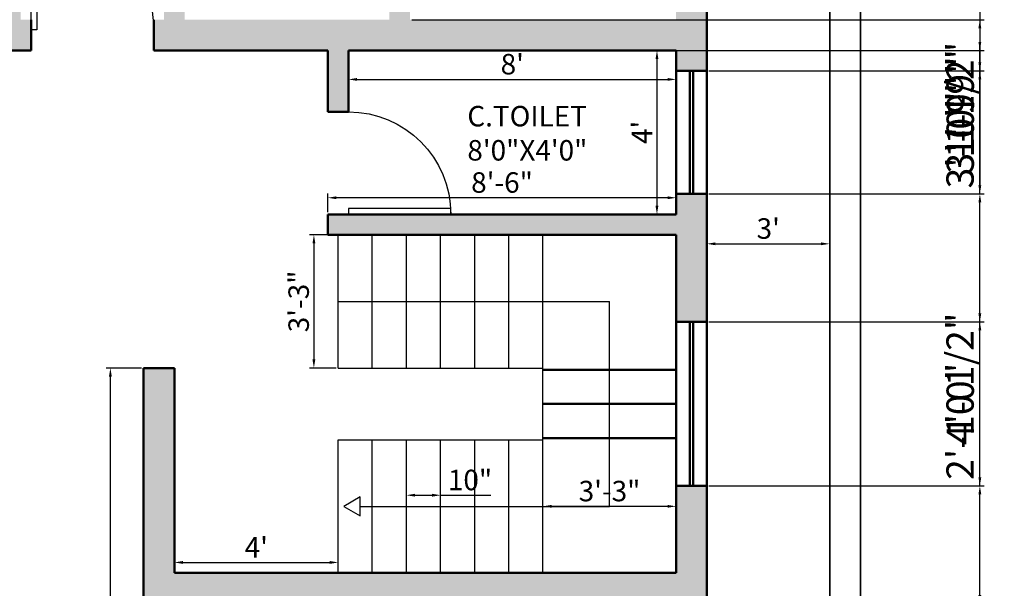
# Model space of a CAD drawing. Units: inches. Extents: x 2442 to 3851, y 589 to 2836.
# Tile 16 of 22: x 2847 to 3136, y 2397 to 2563. Entities that reach past the tile are written whole.
import ezdxf

# ---------------------------------------------------------------- set-up
doc = ezdxf.new("R2010")
doc.units = ezdxf.units.IN
for name, color, linetype, lineweight in [('A-ANNO-DIMS', 2, 'Continuous', 18), ('A-AREA-IDEN', 7, 'Continuous', 18), ('A-DOOR', 4, 'Continuous', 25), ('A-FLOR-STRS', 3, 'Continuous', 25), ('A-WALL', 7, 'Continuous', 50), ('A-WALL-PATT', 8, 'Continuous', 13), ('C-PROP', 7, 'Continuous', 35)]:
    doc.layers.add(name, color=color, linetype=linetype, lineweight=lineweight)
doc.styles.get("Standard").update_dxf_attribs({"font": 'arial.ttf'})
doc.dimstyles.new('ISO-25', dxfattribs={"dimtxt": 8, "dimasz": 2.5, "dimexe": 1.25, "dimexo": 0.625, "dimtad": 1, "dimlunit": 3, "dimtxsty": 'Standard', "dimcen": 2.5, "dimadec": 0, "dimazin": 0, "dimtfac": 1, "dimtmove": 0, "dimatfit": 3, "dimfxl": 1, "dimarcsym": 0})

# ---------------------------------------------------------------- blocks, each defined once
blk = doc.blocks.new('*U23')
for p, q in [((0, 0), (0, -6)), ((36, 0), (36, -6))]:
    blk.add_line(p, q)
blk.add_lwpolyline([(0, 0), (0, 36), (1.75, 36), (1.75, 0)], close=True)
blk.add_arc((0, 0), 36, 0, 90)
blk = doc.blocks.new('*U24')
for p, q in [((0, 0), (0, -6)), ((30, 0), (30, -6))]:
    blk.add_line(p, q)
blk.add_lwpolyline([(0, 0), (0, 30), (1.75, 30), (1.75, 0)], close=True)
blk.add_arc((0, 0), 30, 0, 90)
blk = doc.blocks.new('*D42')
at = {"layer": 'A-ANNO-DIMS', "color": 0, "lineweight": -2, "transparency": 16777216}
for p, q in [((3048.6, 2498.21), (3048.6, 2498.83)), ((3084.6, 2498.21), (3084.6, 2498.83)), ((3051.1, 2497.58), (3082.1, 2497.58))]:
    blk.add_line(p, q, dxfattribs=at)
at = {"layer": 'A-ANNO-DIMS', "color": 0, "transparency": 16777216}
for points in [[(3051.1, 2498), (3051.1, 2497.17), (3048.6, 2497.58)], [(3082.1, 2498), (3082.1, 2497.17), (3084.6, 2497.58)]]:
    blk.add_solid(points, dxfattribs=at)
at = {"layer": 'Defpoints', "color": 0, "transparency": 16777216}
for p in [(3048.6, 2497.58), (3084.6, 2497.58), (3084.6, 2497.58)]:
    blk.add_point(p, dxfattribs=at)
at = {"layer": 'A-ANNO-DIMS', "color": 0, "transparency": 16777216, "insert": (3066.6, 2501.28), "char_height": 6, "attachment_point": 5}
blk.add_mtext("3'", dxfattribs=at)
blk = doc.blocks.new('*D52')
at = {"layer": 'A-ANNO-DIMS', "color": 0, "lineweight": -2, "transparency": 16777216}
for p, q in [((2943.6, 2553.58), (2943.6, 2544.47)), ((3039.6, 2553.58), (3039.6, 2544.47)), ((2946.1, 2545.72), (3037.1, 2545.72))]:
    blk.add_line(p, q, dxfattribs=at)
at = {"layer": 'A-ANNO-DIMS', "color": 0, "transparency": 16777216}
for points in [[(2946.1, 2546.14), (2946.1, 2545.31), (2943.6, 2545.72)], [(3037.1, 2546.14), (3037.1, 2545.31), (3039.6, 2545.72)]]:
    blk.add_solid(points, dxfattribs=at)
at = {"layer": 'Defpoints', "color": 0, "transparency": 16777216}
for p in [(2943.6, 2554.21), (3039.6, 2554.21), (3039.6, 2545.72)]:
    blk.add_point(p, dxfattribs=at)
at = {"layer": 'A-ANNO-DIMS', "color": 0, "transparency": 16777216, "insert": (2991.6, 2549.41), "char_height": 6, "attachment_point": 5}
blk.add_mtext("8'", dxfattribs=at)
blk = doc.blocks.new('*D53')
at = {"layer": 'A-ANNO-DIMS', "color": 0, "lineweight": -2, "transparency": 16777216}
for p, q in [((3038.97, 2554.21), (3032.75, 2554.21)), ((3034, 2551.71), (3034, 2508.71)), ((3038.97, 2506.21), (3032.75, 2506.21))]:
    blk.add_line(p, q, dxfattribs=at)
at = {"layer": 'A-ANNO-DIMS', "color": 0, "transparency": 16777216}
for points in [[(3033.58, 2551.71), (3034.41, 2551.71), (3034, 2554.21)], [(3033.58, 2508.71), (3034.41, 2508.71), (3034, 2506.21)]]:
    blk.add_solid(points, dxfattribs=at)
at = {"layer": 'Defpoints', "color": 0, "transparency": 16777216}
for p in [(3039.6, 2554.21), (3034, 2506.21), (3039.6, 2506.21)]:
    blk.add_point(p, dxfattribs=at)
at = {"layer": 'A-ANNO-DIMS', "color": 0, "transparency": 16777216, "insert": (3030.37, 2530.21), "char_height": 6, "attachment_point": 5, "rotation": 90}
blk.add_mtext("4'", dxfattribs=at)
blk = doc.blocks.new('*D55')
at = {"layer": 'A-ANNO-DIMS', "color": 0, "lineweight": -2, "transparency": 16777216}
for p, q in [((2882.97, 2461.21), (2872.6, 2461.21)), ((2873.85, 2259.71), (2873.85, 2458.71)), ((2882.97, 2257.21), (2872.6, 2257.21))]:
    blk.add_line(p, q, dxfattribs=at)
at = {"layer": 'A-ANNO-DIMS', "color": 0, "transparency": 16777216}
for points in [[(2873.44, 2458.71), (2874.27, 2458.71), (2873.85, 2461.21)], [(2873.44, 2259.71), (2874.27, 2259.71), (2873.85, 2257.21)]]:
    blk.add_solid(points, dxfattribs=at)
at = {"layer": 'Defpoints', "color": 0, "transparency": 16777216}
for p in [(2873.85, 2461.21), (2883.6, 2461.21), (2883.6, 2257.21)]:
    blk.add_point(p, dxfattribs=at)
at = {"layer": 'A-ANNO-DIMS', "color": 0, "transparency": 16777216, "insert": (2870.22, 2359.21), "char_height": 6, "attachment_point": 5, "rotation": 90}
blk.add_mtext("17'", dxfattribs=at)
blk = doc.blocks.new('*D68')
at = {"layer": 'A-ANNO-DIMS', "color": 0, "lineweight": -2, "transparency": 16777216}
for p, q in [((2937.6, 2506.83), (2937.6, 2512.32)), ((3037.1, 2511.07), (2940.1, 2511.07)), ((3039.6, 2506.83), (3039.6, 2512.32))]:
    blk.add_line(p, q, dxfattribs=at)
at = {"layer": 'A-ANNO-DIMS', "color": 0, "transparency": 16777216}
for points in [[(2940.1, 2511.49), (2940.1, 2510.65), (2937.6, 2511.07)], [(3037.1, 2511.49), (3037.1, 2510.65), (3039.6, 2511.07)]]:
    blk.add_solid(points, dxfattribs=at)
at = {"layer": 'Defpoints', "color": 0, "transparency": 16777216}
for p in [(2937.6, 2511.07), (2937.6, 2506.21), (3039.6, 2506.21)]:
    blk.add_point(p, dxfattribs=at)
at = {"layer": 'A-ANNO-DIMS', "color": 0, "transparency": 16777216, "insert": (2988.6, 2514.76), "char_height": 6, "attachment_point": 5}
blk.add_mtext('8\'-6"', dxfattribs=at)
blk = doc.blocks.new('*D69')
at = {"layer": 'A-ANNO-DIMS', "color": 0, "lineweight": -2, "transparency": 16777216}
for p, q in [((2892.6, 2401.83), (2892.6, 2405.53)), ((2895.1, 2404.28), (2938.1, 2404.28)), ((2940.6, 2401.83), (2940.6, 2405.53))]:
    blk.add_line(p, q, dxfattribs=at)
at = {"layer": 'A-ANNO-DIMS', "color": 0, "transparency": 16777216}
for points in [[(2895.1, 2404.7), (2895.1, 2403.86), (2892.6, 2404.28)], [(2938.1, 2404.7), (2938.1, 2403.86), (2940.6, 2404.28)]]:
    blk.add_solid(points, dxfattribs=at)
at = {"layer": 'Defpoints', "color": 0, "transparency": 16777216}
for p in [(2940.6, 2404.28), (2892.6, 2401.21), (2940.6, 2401.21)]:
    blk.add_point(p, dxfattribs=at)
at = {"layer": 'A-ANNO-DIMS', "color": 0, "transparency": 16777216, "insert": (2916.6, 2407.91), "char_height": 6, "attachment_point": 5}
blk.add_mtext("4'", dxfattribs=at)
blk = doc.blocks.new('*D70')
at = {"layer": 'A-ANNO-DIMS', "color": 0, "lineweight": -2, "transparency": 16777216}
for p, q in [((2939.97, 2500.21), (2932.23, 2500.21)), ((2933.48, 2497.71), (2933.48, 2463.71)), ((2939.97, 2461.21), (2932.23, 2461.21))]:
    blk.add_line(p, q, dxfattribs=at)
at = {"layer": 'A-ANNO-DIMS', "color": 0, "transparency": 16777216}
for points in [[(2933.06, 2497.71), (2933.9, 2497.71), (2933.48, 2500.21)], [(2933.06, 2463.71), (2933.9, 2463.71), (2933.48, 2461.21)]]:
    blk.add_solid(points, dxfattribs=at)
at = {"layer": 'Defpoints', "color": 0, "transparency": 16777216}
for p in [(2940.6, 2500.21), (2933.48, 2461.21), (2940.6, 2461.21)]:
    blk.add_point(p, dxfattribs=at)
at = {"layer": 'A-ANNO-DIMS', "color": 0, "transparency": 16777216, "insert": (2929.79, 2480.71), "char_height": 6, "attachment_point": 5, "rotation": 90}
blk.add_mtext('3\'-3"', dxfattribs=at)
blk = doc.blocks.new('*D71')
at = {"layer": 'A-ANNO-DIMS', "color": 0, "lineweight": -2, "transparency": 16777216}
for p, q in [((3000.6, 2421.33), (3000.6, 2421.96)), ((3003.1, 2420.71), (3037.1, 2420.71)), ((3039.6, 2421.33), (3039.6, 2421.96))]:
    blk.add_line(p, q, dxfattribs=at)
at = {"layer": 'A-ANNO-DIMS', "color": 0, "transparency": 16777216}
for points in [[(3003.1, 2421.12), (3003.1, 2420.29), (3000.6, 2420.71)], [(3037.1, 2421.12), (3037.1, 2420.29), (3039.6, 2420.71)]]:
    blk.add_solid(points, dxfattribs=at)
at = {"layer": 'Defpoints', "color": 0, "transparency": 16777216}
for p in [(3000.6, 2420.71), (3039.6, 2420.71), (3039.6, 2420.71)]:
    blk.add_point(p, dxfattribs=at)
at = {"layer": 'A-ANNO-DIMS', "color": 0, "transparency": 16777216, "insert": (3020.1, 2424.4), "char_height": 6, "attachment_point": 5}
blk.add_mtext('3\'-3"', dxfattribs=at)
blk = doc.blocks.new('*D72')
at = {"layer": 'A-ANNO-DIMS', "color": 0, "lineweight": -2, "transparency": 16777216}
for p, q in [((2960.6, 2424.59), (2960.6, 2425.21)), ((2963.1, 2423.96), (2968.1, 2423.96)), ((2970.6, 2424.59), (2970.6, 2425.21)), ((2970.6, 2423.96), (2985.34, 2423.96))]:
    blk.add_line(p, q, dxfattribs=at)
at = {"layer": 'A-ANNO-DIMS', "color": 0, "transparency": 16777216}
for points in [[(2963.1, 2424.38), (2963.1, 2423.55), (2960.6, 2423.96)], [(2968.1, 2424.38), (2968.1, 2423.55), (2970.6, 2423.96)]]:
    blk.add_solid(points, dxfattribs=at)
at = {"layer": 'Defpoints', "color": 0, "transparency": 16777216}
for p in [(2960.6, 2423.96), (2970.6, 2423.96), (2970.6, 2423.96)]:
    blk.add_point(p, dxfattribs=at)
at = {"layer": 'A-ANNO-DIMS', "color": 0, "transparency": 16777216, "insert": (2979.22, 2427.65), "char_height": 6, "attachment_point": 5}
blk.add_mtext('10"', dxfattribs=at)
blk = doc.blocks.new('*D191')
at = {"layer": 'A-ANNO-DIMS', "color": 0, "lineweight": -2, "transparency": 16777216}
for p, q in [((3128.6, 2426.71), (3128.6, 2476.72)), ((3049.22, 2426.71), (3129.85, 2426.71)), ((3128.6, 2394.71), (3128.6, 2424.21)), ((3049.22, 2392.21), (3129.85, 2392.21))]:
    blk.add_line(p, q, dxfattribs=at)
at = {"layer": 'A-ANNO-DIMS', "color": 0, "transparency": 16777216}
for points in [[(3128.18, 2424.21), (3129.02, 2424.21), (3128.6, 2426.71)], [(3128.18, 2394.71), (3129.02, 2394.71), (3128.6, 2392.21)]]:
    blk.add_solid(points, dxfattribs=at)
at = {"layer": 'Defpoints', "color": 0, "transparency": 16777216}
for p in [(3048.6, 2426.71), (3128.6, 2426.71), (3048.6, 2392.21)]:
    blk.add_point(p, dxfattribs=at)
at = {"layer": 'A-ANNO-DIMS', "color": 0, "transparency": 16777216, "insert": (3123.84, 2452.96), "char_height": 8, "attachment_point": 5, "rotation": 90}
blk.add_mtext('2\'-10 1/2"', dxfattribs=at)
blk = doc.blocks.new('*D192')
at = {"layer": 'A-ANNO-DIMS', "color": 0, "lineweight": -2, "transparency": 16777216}
for p, q in [((3049.22, 2474.71), (3129.85, 2474.71)), ((3128.6, 2429.21), (3128.6, 2472.21)), ((3049.22, 2426.71), (3129.85, 2426.71))]:
    blk.add_line(p, q, dxfattribs=at)
at = {"layer": 'A-ANNO-DIMS', "color": 0, "transparency": 16777216}
for points in [[(3128.18, 2472.21), (3129.02, 2472.21), (3128.6, 2474.71)], [(3128.18, 2429.21), (3129.02, 2429.21), (3128.6, 2426.71)]]:
    blk.add_solid(points, dxfattribs=at)
at = {"layer": 'Defpoints', "color": 0, "transparency": 16777216}
for p in [(3048.6, 2474.71), (3128.6, 2474.71), (3048.6, 2426.71)]:
    blk.add_point(p, dxfattribs=at)
at = {"layer": 'A-ANNO-DIMS', "color": 0, "transparency": 16777216, "insert": (3123.89, 2450.71), "char_height": 8, "attachment_point": 5, "rotation": 90}
blk.add_mtext('4\'-0"', dxfattribs=at)
blk = doc.blocks.new('*D193')
at = {"layer": 'A-ANNO-DIMS', "color": 0, "lineweight": -2, "transparency": 16777216}
for p, q in [((3128.6, 2512.21), (3128.6, 2555.86)), ((3049.22, 2512.21), (3129.85, 2512.21)), ((3128.6, 2477.21), (3128.6, 2509.71)), ((3049.22, 2474.71), (3129.85, 2474.71))]:
    blk.add_line(p, q, dxfattribs=at)
at = {"layer": 'A-ANNO-DIMS', "color": 0, "transparency": 16777216}
for points in [[(3128.18, 2509.71), (3129.02, 2509.71), (3128.6, 2512.21)], [(3128.18, 2477.21), (3129.02, 2477.21), (3128.6, 2474.71)]]:
    blk.add_solid(points, dxfattribs=at)
at = {"layer": 'Defpoints', "color": 0, "transparency": 16777216}
for p in [(3048.6, 2512.21), (3128.6, 2512.21), (3048.6, 2474.71)]:
    blk.add_point(p, dxfattribs=at)
at = {"layer": 'A-ANNO-DIMS', "color": 0, "transparency": 16777216, "insert": (3123.83, 2535.28), "char_height": 8, "attachment_point": 5, "rotation": 90}
blk.add_mtext('3\'-1 1/2"', dxfattribs=at)
blk = doc.blocks.new('*D196')
at = {"layer": 'A-ANNO-DIMS', "color": 0, "lineweight": -2, "transparency": 16777216}
for p, q in [((3049.22, 2569.21), (3129.85, 2569.21)), ((3128.6, 2566.71), (3128.6, 2550.71)), ((3049.22, 2548.21), (3129.85, 2548.21)), ((3128.6, 2548.21), (3128.6, 2523.94))]:
    blk.add_line(p, q, dxfattribs=at)
at = {"layer": 'A-ANNO-DIMS', "color": 0, "transparency": 16777216}
for points in [[(3128.18, 2566.71), (3129.02, 2566.71), (3128.6, 2569.21)], [(3128.18, 2550.71), (3129.02, 2550.71), (3128.6, 2548.21)]]:
    blk.add_solid(points, dxfattribs=at)
at = {"layer": 'Defpoints', "color": 0, "transparency": 16777216}
for p in [(3048.6, 2569.21), (3048.6, 2548.21), (3128.6, 2548.21)]:
    blk.add_point(p, dxfattribs=at)
at = {"layer": 'A-ANNO-DIMS', "color": 0, "transparency": 16777216, "insert": (3123.89, 2534.83), "char_height": 8, "attachment_point": 5, "rotation": 90}
blk.add_mtext('1\'-9"', dxfattribs=at)
blk = doc.blocks.new('*D197')
at = {"layer": 'A-ANNO-DIMS', "color": 0, "lineweight": -2, "transparency": 16777216}
for p, q in [((3049.22, 2548.21), (3129.85, 2548.21)), ((3128.6, 2545.71), (3128.6, 2514.71)), ((3049.22, 2512.21), (3129.85, 2512.21))]:
    blk.add_line(p, q, dxfattribs=at)
at = {"layer": 'A-ANNO-DIMS', "color": 0, "transparency": 16777216}
for points in [[(3128.18, 2545.71), (3129.02, 2545.71), (3128.6, 2548.21)], [(3128.18, 2514.71), (3129.02, 2514.71), (3128.6, 2512.21)]]:
    blk.add_solid(points, dxfattribs=at)
at = {"layer": 'Defpoints', "color": 0, "transparency": 16777216}
for p in [(3048.6, 2548.21), (3048.6, 2512.21), (3128.6, 2512.21)]:
    blk.add_point(p, dxfattribs=at)
at = {"layer": 'A-ANNO-DIMS', "color": 0, "transparency": 16777216, "insert": (3123.89, 2530.21), "char_height": 8, "attachment_point": 5, "rotation": 90}
blk.add_mtext('3\'-0"', dxfattribs=at)
blk = doc.blocks.new('*D215')
at = {"layer": 'A-ANNO-DIMS', "color": 0, "lineweight": -2, "transparency": 16777216}
for p, q in [((2962.22, 2563.21), (3129.85, 2563.21)), ((3128.6, 2560.71), (3128.6, 2556.71)), ((2944.22, 2554.21), (3129.85, 2554.21)), ((3128.6, 2554.21), (3128.6, 2529.19))]:
    blk.add_line(p, q, dxfattribs=at)
at = {"layer": 'A-ANNO-DIMS', "color": 0, "transparency": 16777216}
for points in [[(3128.18, 2560.71), (3129.02, 2560.71), (3128.6, 2563.21)], [(3128.18, 2556.71), (3129.02, 2556.71), (3128.6, 2554.21)]]:
    blk.add_solid(points, dxfattribs=at)
at = {"layer": 'Defpoints', "color": 0, "transparency": 16777216}
for p in [(2961.6, 2563.21), (2943.6, 2554.21), (3128.6, 2554.21)]:
    blk.add_point(p, dxfattribs=at)
at = {"layer": 'A-ANNO-DIMS', "color": 0, "transparency": 16777216, "insert": (3123.89, 2540.45), "char_height": 8, "attachment_point": 5, "rotation": 90}
blk.add_mtext('0\'-9"', dxfattribs=at)

msp = doc.modelspace()

# ---------------------------------------------------------------- hatches: boundary and pattern name
at = {"layer": 'A-WALL-PATT'}
h = msp.add_hatch(color=256, dxfattribs=at)
h.dxf.hatch_style = 1
h.paths.add_polyline_path([(2640.599, 2713.208), (2640.599, 2719.208), (2640.599, 2722.208), (2538.599, 2722.208), (2538.599, 2657.708), (2547.599, 2657.708), (2547.599, 2713.208)])
h.paths.add_polyline_path([(2700.599, 2737.208), (2730.599, 2737.208), (2730.599, 2746.208), (2700.599, 2746.208), (2700.599, 2782.208), (2691.599, 2782.208), (2691.599, 2722.208), (2670.599, 2722.208), (2670.599, 2719.208), (2670.599, 2713.208), (2691.599, 2713.208), (2691.599, 2608.208), (2799.599, 2608.208), (2799.599, 2614.208), (2799.599, 2617.208), (2700.599, 2617.208)])
h.paths.add_polyline_path([(2838.599, 2737.208), (2838.599, 2617.208), (2835.599, 2617.208), (2835.599, 2614.208), (2835.599, 2608.208), (2838.599, 2608.208), (2838.599, 2554.208), (2850.599, 2554.208), (2850.599, 2560.208), (2850.599, 2563.208), (2847.599, 2563.208), (2847.599, 2737.208), (2850.599, 2737.208), (2850.599, 2746.208), (2796.599, 2746.208), (2796.599, 2737.208)])
h.paths.add_polyline_path([(2898.599, 2746.208), (2898.599, 2737.208), (2967.599, 2737.208), (2967.599, 2746.208)])
h.paths.add_polyline_path([(3048.599, 2746.208), (3015.599, 2746.208), (3015.599, 2737.208), (3039.599, 2737.208), (3039.599, 2665.208), (3048.599, 2665.208)])
h.paths.add_polyline_path([(3039.599, 2611.208), (3039.599, 2605.208), (3048.599, 2605.208), (3048.599, 2617.208), (2946.599, 2617.208), (2946.599, 2611.208)])
h.paths.add_polyline_path([(2961.599, 2563.208), (2961.599, 2581.208), (2955.599, 2581.208), (2955.599, 2563.208), (2895.599, 2563.208), (2895.599, 2611.208), (2916.599, 2611.208), (2916.599, 2617.208), (2889.599, 2617.208), (2889.599, 2563.208), (2886.599, 2563.208), (2886.599, 2554.208), (2937.599, 2554.208), (2937.599, 2536.208), (2943.599, 2536.208), (2943.599, 2554.208), (3039.599, 2554.208), (3039.599, 2548.208), (3048.599, 2548.208), (3048.599, 2569.208), (3039.599, 2569.208), (3039.599, 2563.208)])
h.paths.add_polyline_path([(2538.599, 2521.208), (2547.599, 2521.208), (2547.599, 2545.208), (2694.599, 2545.208), (2694.599, 2542.208), (2697.599, 2542.208), (2703.599, 2542.208), (2703.599, 2554.208), (2547.599, 2554.208), (2547.599, 2609.708), (2538.599, 2609.708)])
h.paths.add_polyline_path([(2538.599, 2368.208), (2547.599, 2368.208), (2547.599, 2392.208), (2694.599, 2392.208), (2694.599, 2344.208), (2703.599, 2344.208), (2703.599, 2506.208), (2697.599, 2506.208), (2694.599, 2506.208), (2694.599, 2401.208), (2547.599, 2401.208), (2547.599, 2473.208), (2538.599, 2473.208)])
h.paths.add_polyline_path([(2547.599, 2287.208), (2553.599, 2287.208), (2553.599, 2293.208), (2553.599, 2296.208), (2547.599, 2296.208), (2547.599, 2320.208), (2538.599, 2320.208), (2538.599, 2191.208), (2547.599, 2191.208)])
h.paths.add_polyline_path([(2703.599, 2296.208), (2670.599, 2296.208), (2670.599, 2287.208), (2694.599, 2287.208), (2694.599, 2248.208), (2733.599, 2248.208), (2733.599, 2257.208), (2703.599, 2257.208)])
h.paths.add_polyline_path([(2593.599, 2287.208), (2604.599, 2287.208), (2604.599, 2296.208), (2593.599, 2296.208)])
h.paths.add_polyline_path([(2799.599, 2248.208), (2799.599, 2257.208), (2775.599, 2257.208), (2775.599, 2248.208)])
h.paths.add_polyline_path([(2892.599, 2248.208), (2892.599, 2287.208), (2883.599, 2287.208), (2883.599, 2257.208), (2865.599, 2257.208), (2865.599, 2248.208)])
h.paths.add_polyline_path([(2883.599, 2353.208), (2892.599, 2353.208), (2892.599, 2392.208), (3048.599, 2392.208), (3048.599, 2426.708), (3039.599, 2426.708), (3039.599, 2401.208), (2892.599, 2401.208), (2892.599, 2461.208), (2883.599, 2461.208)])
h.paths.add_polyline_path([(3039.599, 2474.708), (3048.599, 2474.708), (3048.599, 2512.208), (3039.599, 2512.208), (3039.599, 2506.208), (2937.599, 2506.208), (2937.599, 2500.208), (3039.599, 2500.208)])

# ---------------------------------------------------------------- linework, layer by layer
at = {"layer": 'A-FLOR-STRS'}
for p, q in [((2940.599, 2461.208), (2940.599, 2500.208)), ((2950.599, 2461.208), (2950.599, 2500.208)), ((2960.599, 2461.208), (2960.599, 2500.208)), ((2970.599, 2461.208), (2970.599, 2500.208)), ((2980.599, 2461.208), (2980.599, 2500.208)), ((2990.599, 2461.208), (2990.599, 2500.208)), ((3000.599, 2440.208), (3000.599, 2500.208)), ((2940.599, 2480.708), (3020.099, 2480.708)), ((3020.099, 2420.708), (3020.099, 2480.708)), ((2940.599, 2461.208), (3000.599, 2461.208)), ((2940.599, 2440.208), (3000.599, 2440.208)), ((2947.056, 2420.708), (3020.099, 2420.708))]:
    msp.add_line(p, q, dxfattribs=at)
at = {"layer": 'A-FLOR-STRS', "ltscale": 0.5}
for p, q in [((2940.599, 2401.208), (2940.599, 2440.208)), ((2950.599, 2401.208), (2950.599, 2440.208)), ((2960.599, 2401.208), (2960.599, 2440.208)), ((2970.599, 2401.208), (2970.599, 2440.208)), ((2980.599, 2401.208), (2980.599, 2440.208)), ((2990.599, 2401.208), (2990.599, 2440.208)), ((3000.599, 2401.208), (3000.599, 2440.208))]:
    msp.add_line(p, q, dxfattribs=at)
at = {"layer": 'A-FLOR-STRS'}
msp.add_lwpolyline([(2942.213, 2420.708), (2947.056, 2417.911), (2947.056, 2423.504)], close=True, dxfattribs=at)
at = {"layer": 'A-WALL'}
for p, q in [((3048.599, 2392.208), (3048.599, 2746.208)), ((2850.599, 2554.208), (2850.599, 2563.208)), ((2886.599, 2554.208), (2886.599, 2563.208)), ((2838.599, 2554.208), (2850.599, 2554.208)), ((2886.599, 2554.208), (2937.599, 2554.208)), ((2937.599, 2536.208), (2937.599, 2554.208)), ((2943.599, 2536.208), (2943.599, 2554.208)), ((2943.599, 2554.208), (3039.599, 2554.208)), ((3039.599, 2506.208), (3039.599, 2554.208)), ((3039.599, 2548.208), (3048.599, 2548.208)), ((3043.599, 2512.208), (3043.599, 2548.208)), ((3044.599, 2512.208), (3044.599, 2548.208)), ((2937.599, 2536.208), (2943.599, 2536.208)), ((3039.599, 2512.208), (3048.599, 2512.208)), ((2937.599, 2500.208), (2937.599, 2506.208)), ((2937.599, 2506.208), (3039.599, 2506.208)), ((2937.599, 2500.208), (3039.599, 2500.208)), ((3039.599, 2401.208), (3039.599, 2500.208)), ((3039.599, 2474.708), (3048.599, 2474.708)), ((3043.599, 2426.708), (3043.599, 2474.708)), ((3044.599, 2426.708), (3044.599, 2474.708)), ((2883.599, 2461.208), (2892.599, 2461.208)), ((2883.599, 2257.208), (2883.599, 2461.208)), ((2892.599, 2401.208), (2892.599, 2461.208)), ((3000.599, 2460.708), (3039.599, 2460.708)), ((3000.599, 2450.708), (3039.599, 2450.708)), ((3000.599, 2440.708), (3039.599, 2440.708)), ((3039.599, 2426.708), (3048.599, 2426.708)), ((2892.599, 2401.208), (3039.599, 2401.208))]:
    msp.add_line(p, q, dxfattribs=at)
at = {"layer": 'C-PROP'}
for points in [[(3066.599, 2191.208), (3093.599, 2191.208), (3093.599, 2791.208), (2493.599, 2791.208), (2493.599, 2191.208), (2738.599, 2191.208)], [(3066.599, 2200.208), (3084.599, 2200.208), (3084.599, 2782.208), (2502.599, 2782.208), (2502.599, 2200.208), (2538.599, 2200.208)]]:
    msp.add_lwpolyline(points, dxfattribs=at)

# ---------------------------------------------------------------- block references
at = {"layer": 'A-DOOR'}
msp.add_blockref('*U23', (2850.599, 2560.208), dxfattribs=at)
at = {"layer": 'A-DOOR', "xscale": -1, "rotation": 270}
msp.add_blockref('*U24', (2943.599, 2506.208), dxfattribs=at)

# ---------------------------------------------------------------- texts
at = {"layer": 'A-AREA-IDEN', "insert": (2978.437, 2537.962), "char_height": 6, "attachment_point": 1}
msp.add_mtext_dynamic_manual_height_columns('{\\fTimes New Roman|b0|i0|c0|p18;C.TOILET\\P8\'0"X4\'0"}', width=110.76054, gutter_width=12.5, heights=[0], dxfattribs=at)

# ---------------------------------------------------------------- dimensions: what is measured, and where the dimension line sits
at = {"layer": 'A-ANNO-DIMS'}
for base, p1, p2, override, picture, middle in [((3128.599, 2548.208), (3048.599, 2569.208), (3048.599, 2548.208), {"dimdec": 1, "dimlfac": 1, "dimrnd": 0, "dimzin": 1, "dimdsep": 46, "dimlunit": 4, "dimfrac": 2}, '*D196', (3123.889, 2534.826)), ((3128.599, 2554.208), (2961.599, 2563.208), (2943.599, 2554.208), {"dimdec": 1, "dimlfac": 1, "dimrnd": 0, "dimzin": 1, "dimdsep": 46, "dimlunit": 4, "dimfrac": 2}, '*D215', (3123.889, 2540.45)), ((3033.995, 2506.208), (3039.599, 2554.208), (3039.599, 2506.208), {"dimtxt": 6, "dimclrd": 0, "dimclre": 0, "dimclrt": 0}, '*D53', (3030.37, 2530.208)), ((3128.599, 2512.208), (3048.599, 2474.708), (3048.599, 2512.208), {"dimdec": 1, "dimlfac": 1, "dimrnd": 0, "dimzin": 1, "dimdsep": 46, "dimlunit": 4, "dimfrac": 2}, '*D193', (3123.835, 2535.283)), ((3128.599, 2512.208), (3048.599, 2548.208), (3048.599, 2512.208), {"dimdec": 1, "dimlfac": 1, "dimrnd": 0, "dimzin": 1, "dimdsep": 46, "dimlunit": 4, "dimfrac": 2}, '*D197', (3123.886, 2530.208)), ((2933.481, 2461.208), (2940.599, 2500.208), (2940.599, 2461.208), {"dimtxt": 6, "dimclrd": 0, "dimclre": 0, "dimclrt": 0}, '*D70', (2929.79, 2480.708)), ((3128.599, 2426.708), (3048.599, 2392.208), (3048.599, 2426.708), {"dimdec": 1, "dimlfac": 1, "dimrnd": 0, "dimzin": 1, "dimdsep": 46, "dimlunit": 4, "dimfrac": 2}, '*D191', (3123.837, 2452.962)), ((3128.599, 2474.708), (3048.599, 2426.708), (3048.599, 2474.708), {"dimdec": 1, "dimlfac": 1, "dimrnd": 0, "dimzin": 1, "dimdsep": 46, "dimlunit": 4, "dimfrac": 2}, '*D192', (3123.889, 2450.708)), ((2873.853, 2461.208), (2883.599, 2257.208), (2883.599, 2461.208), {"dimtxt": 6, "dimclrd": 0, "dimclre": 0, "dimclrt": 0}, '*D55', (2870.216, 2359.208))]:
    dim = msp.add_linear_dim(base=base, p1=p1, p2=p2, angle=90, dimstyle='ISO-25', override=override, dxfattribs=at)
    dim.commit()
    dim.dimension.update_dxf_attribs({"geometry": picture, "text_midpoint": middle})
for base, p1, p2, picture, middle in [((3039.599, 2545.724), (2943.599, 2554.208), (3039.599, 2554.208), '*D52', (2991.599, 2549.412)), ((2937.599, 2511.07), (3039.599, 2506.208), (2937.599, 2506.208), '*D68', (2988.599, 2514.758)), ((3084.599, 2497.585), (3048.599, 2497.585), (3084.599, 2497.585), '*D42', (3066.599, 2501.275)), ((2970.599, 2423.962), (2960.599, 2423.962), (2970.599, 2423.962), '*D72', (2979.22, 2427.651)), ((3039.599, 2420.708), (3000.599, 2420.708), (3039.599, 2420.708), '*D71', (3020.099, 2424.398)), ((2940.599, 2404.28), (2892.599, 2401.208), (2940.599, 2401.208), '*D69', (2916.599, 2407.905))]:
    dim = msp.add_linear_dim(base=base, p1=p1, p2=p2, dimstyle='ISO-25', override={"dimtxt": 6, "dimclrd": 0, "dimclre": 0, "dimclrt": 0}, dxfattribs=at)
    dim.commit()
    dim.dimension.update_dxf_attribs({"geometry": picture, "text_midpoint": middle})

doc.saveas('drawing.dxf')
